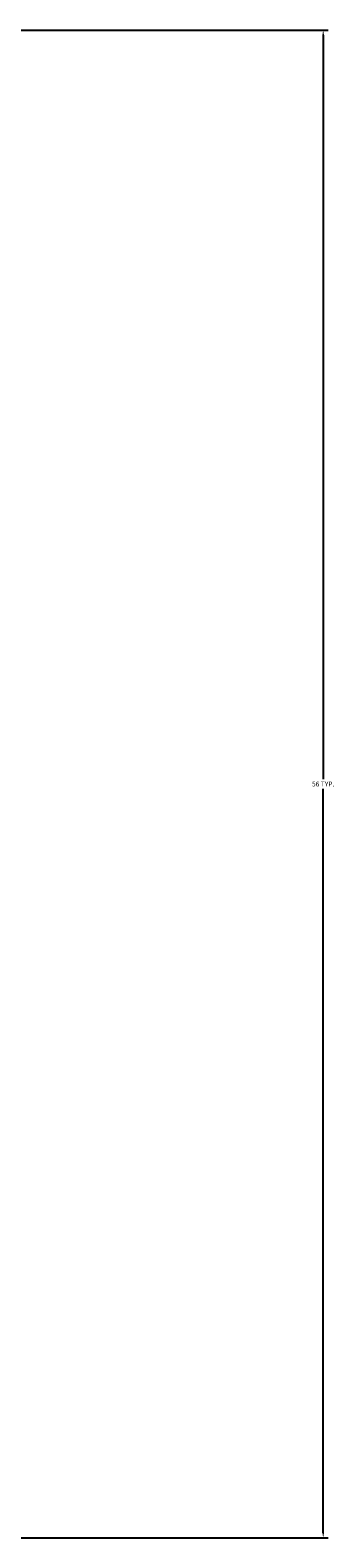
# Model space of a CAD drawing. Units: inches. Extents: x 2168 to 3056, y 1130 to 2629.
# Tile 29 of 42: x 2549 to 2560, y 2320 to 2376. Entities that reach past the tile are written whole.
import ezdxf

# ---------------------------------------------------------------- set-up
doc = ezdxf.new("R2010")
doc.units = ezdxf.units.IN
doc.layers.add('A-ANNO-DIMS', color=2, linetype='Continuous', lineweight=18)
doc.styles.get("Standard").update_dxf_attribs({"font": 'arial.ttf'})
doc.dimstyles.get("Standard").update_dxf_attribs({"dimtxt": 0.18, "dimasz": 0.18, "dimexe": 0.18, "dimexo": 0.0625, "dimgap": 0.09, "dimtad": 0, "dimtih": 1, "dimtoh": 1, "dimdec": 4, "dimzin": 0, "dimdsep": 46, "dimtxsty": 'Standard', "dimcen": 0.09, "dimadec": 0, "dimazin": 0, "dimtfac": 1, "dimtdec": 4, "dimtofl": 0, "dimtmove": 0, "dimatfit": 3, "dimfxl": 1, "dimtolj": 1, "dimtzin": 0, "dimarcsym": 0})

# ---------------------------------------------------------------- blocks, each defined once
blk = doc.blocks.new('*D15')
at = {"layer": 'A-ANNO-DIMS', "color": 0, "lineweight": -2, "transparency": 16777216}
for p, q in [((2547.835, 2375.76), (2560.185, 2375.76)), ((2560.005, 2375.58), (2560.005, 2348.029)), ((2560.005, 2320.115), (2560.005, 2347.665)), ((2547.835, 2319.935), (2560.185, 2319.935))]:
    blk.add_line(p, q, dxfattribs=at)
at = {"layer": 'A-ANNO-DIMS', "color": 0, "transparency": 16777216}
for points in [[(2559.975, 2375.58), (2560.035, 2375.58), (2560.005, 2375.76)], [(2559.975, 2320.115), (2560.035, 2320.115), (2560.005, 2319.935)]]:
    blk.add_solid(points, dxfattribs=at)
at = {"layer": 'Defpoints', "color": 0, "transparency": 16777216}
for p in [(2547.772, 2375.76), (2560.005, 2375.76), (2547.772, 2319.935)]:
    blk.add_point(p, dxfattribs=at)
at = {"layer": 'A-ANNO-DIMS', "color": 0, "transparency": 16777216, "insert": (2560.005, 2347.847), "char_height": 0.18, "attachment_point": 5}
blk.add_mtext('\\A1;56 TYP.', dxfattribs=at)

msp = doc.modelspace()

# ---------------------------------------------------------------- dimensions: what is measured, and where the dimension line sits
at = {"layer": 'A-ANNO-DIMS'}
dim = msp.add_linear_dim(base=(2560.005, 2375.76), p1=(2547.772, 2319.935), p2=(2547.772, 2375.76), angle=90, text='<> TYP.', dimstyle='Standard', override={"dimdec": 0, "dimlfac": 1, "dimrnd": 0, "dimzin": 0, "dimdsep": 46, "dimlunit": 2}, dxfattribs=at)
dim.commit()
dim.dimension.update_dxf_attribs({"geometry": '*D15', "text_midpoint": (2560.005, 2347.847)})

doc.saveas('drawing.dxf')
